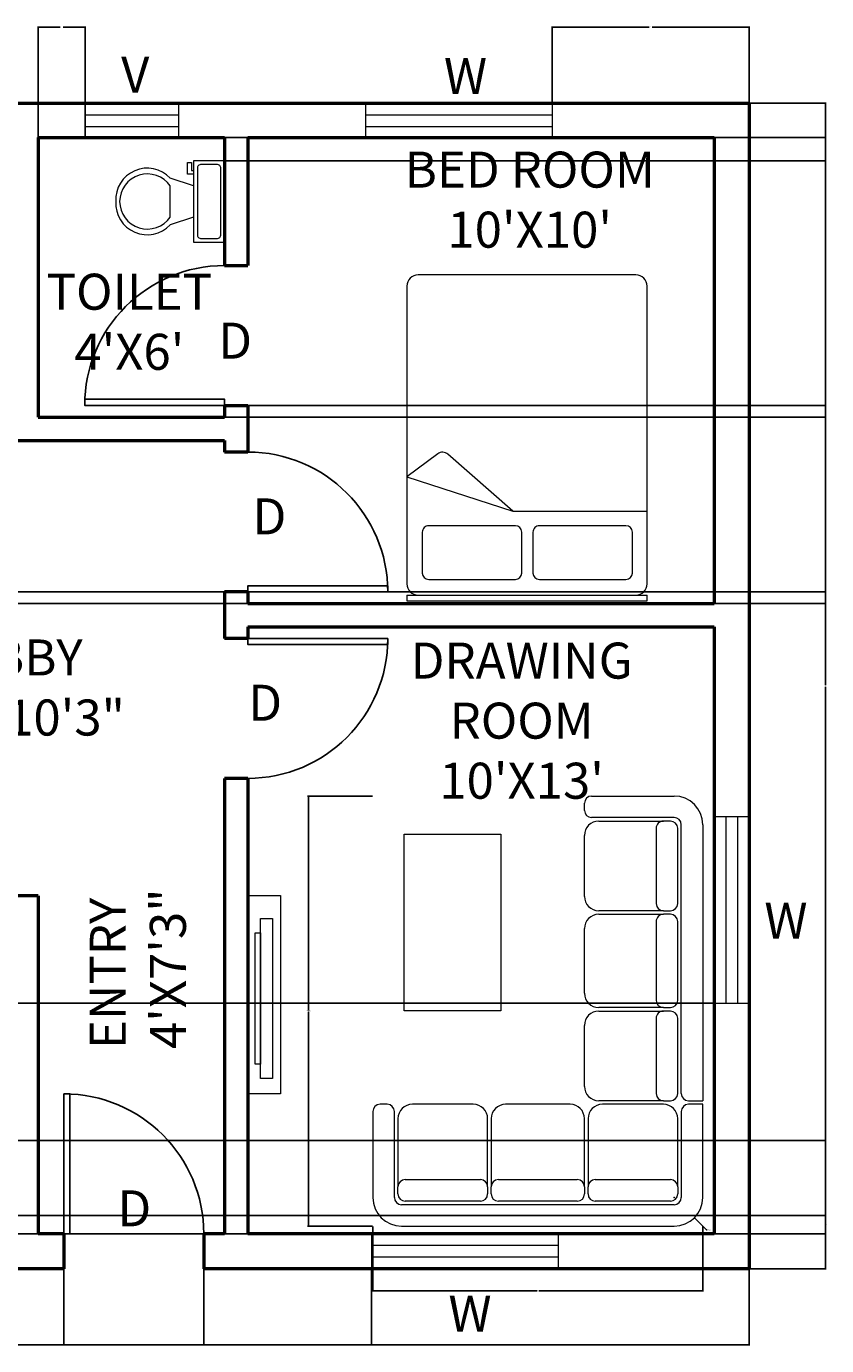
# Model space of a CAD drawing. Units: inches. Extents: x 1916 to 2328, y 785 to 1125.
# Tile 3 of 3: x 2122 to 2328, y 785 to 1125. Entities that reach past the tile are written whole.
import ezdxf

# ---------------------------------------------------------------- set-up
doc = ezdxf.new("R2010")
doc.units = ezdxf.units.IN
for name, color, linetype, lineweight in [('A-ANNO-DIMS', 2, 'Continuous', 18), ('A-ANNO-TEXT', 7, 'Continuous', 18), ('A-AREA-IDEN', 7, 'Continuous', 25), ('A-DOOR', 3, 'Continuous', 25), ('A-FLOR-FIXT', 9, 'Continuous', 18), ('A-FURN', 8, 'Continuous', 18), ('A-GLAZ', 4, 'Continuous', 18), ('A-WALL', 7, 'Continuous', 50)]:
    doc.layers.add(name, color=color, linetype=linetype, lineweight=lineweight)
doc.styles.get("Standard").update_dxf_attribs({"font": 'arial.ttf'})
doc.dimstyles.get("Standard").update_dxf_attribs({"dimtxt": 0.18, "dimasz": 0.18, "dimexe": 0.18, "dimexo": 0.0625, "dimgap": 0.09, "dimtad": 0, "dimtih": 1, "dimtoh": 1, "dimdec": 4, "dimzin": 0, "dimdsep": 46, "dimtxsty": 'Standard', "dimcen": 0.09, "dimadec": 0, "dimazin": 0, "dimtfac": 1, "dimtdec": 4, "dimtofl": 0, "dimtmove": 0, "dimatfit": 3, "dimfxl": 1, "dimtolj": 1, "dimtzin": 0, "dimarcsym": 0})

# ---------------------------------------------------------------- blocks, each defined once
blk = doc.blocks.new('*U2')
for p, q in [((0, 0), (0, -6)), ((40, 0), (40, -6))]:
    blk.add_line(p, q)
blk.add_lwpolyline([(0, 0), (0, 40), (1.75, 40), (1.75, 0)], close=True)
blk.add_arc((0, 0), 40, 0, 90)
blk = doc.blocks.new('*U3')
for p, q in [((0, 0), (0, 6)), ((40, 0), (40, 6))]:
    blk.add_line(p, q)
blk.add_lwpolyline([(0, 0), (0, -40), (1.75, -40), (1.75, 0)], close=True)
blk.add_arc((0, 0), 40, 270, 0)
blk = doc.blocks.new('A$C2AFA021D')
for p, q in [((0.8, 2.3), (0.2, 2.3)), ((0.85, 2.2), (0.85, 2.25)), ((0.2, 2.15), (0.8, 2.15)), ((0.225, 2.125), (0.275, 2.125)), ((0.75, 2.125), (0.275, 2.125)), ((0, 2.1), (0, 0.2)), ((0.15, 0.2), (0.15, 2.1)), ((0.175, 1.55), (0.175, 2.075)), ((0.325, 2.075), (0.325, 1.55)), ((0.85, 1.6), (0.85, 2.025)), ((0.275, 1.5), (0.225, 1.5)), ((0.225, 1.475), (0.275, 1.475)), ((0.275, 1.5), (0.75, 1.5)), ((0.75, 1.475), (0.275, 1.475)), ((0.175, 0.875), (0.175, 1.425)), ((0.325, 1.425), (0.325, 0.875)), ((0.85, 0.925), (0.85, 1.375)), ((0.175, 0.225), (0.175, 0.75)), ((0.275, 0.825), (0.225, 0.825)), ((0.225, 0.8), (0.275, 0.8)), ((0.275, 0.825), (0.75, 0.825)), ((0.75, 0.8), (0.275, 0.8)), ((0.325, 0.75), (0.325, 0.225)), ((0.975, 0.825), (1.4, 0.825)), ((1.625, 0.825), (2.075, 0.825)), ((2.3, 0.825), (2.725, 0.825)), ((2.85, 0.2), (2.85, 0.775)), ((2.9, 0.825), (2.95, 0.825)), ((3, 0.775), (3, 0.2)), ((0.85, 0.275), (0.85, 0.7)), ((0.875, 0.275), (0.875, 0.725)), ((1.5, 0.725), (1.5, 0.275)), ((1.525, 0.275), (1.525, 0.725)), ((2.175, 0.725), (2.175, 0.275)), ((2.2, 0.275), (2.2, 0.725)), ((2.825, 0.725), (2.825, 0.275)), ((1.45, 0.325), (0.925, 0.325)), ((2.125, 0.325), (1.575, 0.325)), ((2.775, 0.325), (2.25, 0.325)), ((0.875, 0.275), (0.875, 0.225)), ((1.5, 0.225), (1.5, 0.275)), ((1.525, 0.275), (1.525, 0.225)), ((2.175, 0.225), (2.175, 0.275)), ((2.2, 0.275), (2.2, 0.225)), ((2.825, 0.225), (2.825, 0.275)), ((0.8, 0.15), (0.2, 0.15)), ((0.275, 0.175), (0.225, 0.175)), ((0.275, 0.175), (0.75, 0.175)), ((0.85, 0), (0.85, 0.1)), ((0.875, 0.1), (0.875, 0)), ((0.925, 0.175), (1.45, 0.175)), ((0.925, 0.15), (2.8, 0.15)), ((1.575, 0.175), (2.125, 0.175)), ((2.25, 0.175), (2.775, 0.175)), ((0.2, 0), (0.85, 0)), ((2.8, 0), (0.875, 0))]:
    blk.add_line(p, q)
for centre, radius, start, end in [((0.2, 2.1), 0.2, 90, 180), ((0.8, 2.25), 0.05, 0, 90), ((0.2, 2.1), 0.05, 90, 180), ((0.225, 2.075), 0.05, 90, 180), ((0.275, 2.075), 0.05, 0, 90), ((0.75, 2.025), 0.1, 0, 90), ((0.8, 2.2), 0.05, 270, 0), ((0.75, 1.6), 0.1, 270, 0), ((0.225, 1.55), 0.05, 180, 270), ((0.225, 1.425), 0.05, 90, 180), ((0.275, 1.55), 0.05, 270, 0), ((0.275, 1.425), 0.05, 0, 90), ((0.75, 1.375), 0.1, 360, 90), ((0.75, 0.925), 0.1, 270, 0), ((0.225, 0.875), 0.05, 180, 270), ((0.275, 0.875), 0.05, 270, 0), ((0.225, 0.75), 0.05, 90, 180), ((0.275, 0.75), 0.05, 0, 90), ((0.75, 0.7), 0.1, 0, 90), ((0.975, 0.725), 0.1, 90, 180), ((1.4, 0.725), 0.1, 0, 90), ((1.625, 0.725), 0.1, 90, 180), ((2.075, 0.725), 0.1, 0, 90), ((2.3, 0.725), 0.1, 90, 180), ((2.725, 0.725), 0.1, 0, 90), ((2.9, 0.775), 0.05, 90, 180), ((2.95, 0.775), 0.05, 0, 90), ((0.925, 0.275), 0.05, 90, 180), ((1.45, 0.275), 0.05, 360, 90), ((1.575, 0.275), 0.05, 90, 180), ((2.125, 0.275), 0.05, 360, 90), ((2.25, 0.275), 0.05, 90, 180), ((2.775, 0.275), 0.05, 360, 90), ((0.2, 0.2), 0.2, 180, 270), ((0.2, 0.2), 0.05, 180, 270), ((0.225, 0.225), 0.05, 180, 270), ((0.275, 0.225), 0.05, 270, 0), ((0.75, 0.275), 0.1, 270, 0), ((0.925, 0.225), 0.05, 180, 270), ((1.45, 0.225), 0.05, 270, 0), ((1.575, 0.225), 0.05, 180, 270), ((2.125, 0.225), 0.05, 270, 0), ((2.25, 0.225), 0.05, 180, 270), ((2.775, 0.225), 0.05, 270, 0), ((2.8, 0.2), 0.2, 270, 0), ((2.8, 0.2), 0.05, 270, 0), ((0.8, 0.1), 0.05, 0, 90), ((0.925, 0.1), 0.05, 90, 180)]:
    blk.add_arc(centre, radius, start, end)
blk = doc.blocks.new('A$C164346CA')
for p, q in [((0, 2.035), (0, 2)), ((1.5, 2.035), (0, 2.035)), ((1.5, 2), (0, 2)), ((1.5, 2), (1.5, 2.035)), ((0, 1.93), (0, 0.07)), ((0.6731, 1.9024), (0.1319, 1.9024)), ((1.364, 1.9024), (0.8228, 1.9024)), ((1.5, 0.07), (1.5, 1.93)), ((0.0919, 1.8624), (0.0919, 1.6069)), ((0.7131, 1.6069), (0.7131, 1.8624)), ((0.7828, 1.8624), (0.7828, 1.6069)), ((1.404, 1.6069), (1.404, 1.8624)), ((0.1319, 1.5669), (0.6731, 1.5669)), ((0.8228, 1.5669), (1.364, 1.5669)), ((0.8395, 1.4761), (0, 1.4761)), ((0.8395, 1.4761), (1.2448, 1.12)), ((1.5, 1.2611), (0.8395, 1.4761)), ((1.3077, 1.1175), (1.5, 1.2611)), ((0.07, 0), (1.43, 0))]:
    blk.add_line(p, q)
for centre, radius, start, end in [((0.07, 1.93), 0.07, 90, 180), ((1.43, 1.93), 0.07, 0, 90), ((0.1319, 1.8624), 0.04, 90, 180), ((0.6731, 1.8624), 0.04, 0, 90), ((0.8228, 1.8624), 0.04, 90, 180), ((1.364, 1.8624), 0.04, 0, 90), ((0.1319, 1.6069), 0.04, 180, 270), ((0.6731, 1.6069), 0.04, 270, 0), ((0.8228, 1.6069), 0.04, 180, 270), ((1.364, 1.6069), 0.04, 270, 0), ((1.2778, 1.1575), 0.05, 228.69584, 306.75789), ((0.07, 0.07), 0.07, 180, 270), ((1.43, 0.07), 0.07, 270, 0)]:
    blk.add_arc(centre, radius, start, end)
blk = doc.blocks.new('*U10')
for p, q in [((9.5, -6), (9.5, -2)), ((-10, -8.5), (-8, -8.5)), ((-10, -9.5), (-10, -8.5)), ((-7, -9.5), (-10, -9.5)), ((-8, -8.5), (-8, -8)), ((-7, -8), (-7, -9.5)), ((-4, -8), (-6, -14)), ((4, -8), (6, -14)), ((4, -14), (-4, -14))]:
    blk.add_line(p, q)
blk.add_lwpolyline([(10.5, -8), (10.5, 0), (-10.5, 0), (-10.5, -8)], close=True)
for points in [[(-9.5, -2), (-9.5, -6)], [(8.5, -1), (-8.5, -1)], [(-8.5, -7), (8.5, -7)]]:
    blk.add_lwpolyline(points)
for centre, radius, start, end in [((-8.625, -1.875), 0.8839, 81.8699, 188.1301), ((8.625, -1.875), 0.8839, 351.8699, 98.1301), ((-8.625, -6.125), 0.8839, 171.869898, 278.1301), ((8.625, -6.125), 0.8839, 261.8699, 8.1301), ((-0.4772, -19.9188), 8.0953, 133.01722, 273.38), ((0.0374, -19.8731), 7.127, 124.50543, 269.7), ((-0.0373, -19.8731), 7.127, 270.3, 55.4946), ((0.4773, -19.9188), 8.0953, 266.62, 46.9828)]:
    blk.add_arc(centre, radius, start, end)
blk = doc.blocks.new('WIN-48-JAMB-9')
for p, q in [((0, 9), (0, 0)), ((48, 9), (48, 0)), ((48, 6), (0, 6)), ((48, 3), (0, 3))]:
    blk.add_line(p, q)
blk = doc.blocks.new('WIN-48-JAMB-8_78')
for p, q in [((0, 8.78), (0, 0)), ((48, 8.78), (48, 0)), ((0, 5.78), (48, 5.78)), ((0, 2.78), (48, 2.78))]:
    blk.add_line(p, q)
blk = doc.blocks.new('VENT-24')
for p, q in [((0, 8.78), (0, 0)), ((24, 8.78), (24, 0)), ((0, 5.78), (24, 5.78)), ((0, 2.78), (24, 2.78))]:
    blk.add_line(p, q)
blk = doc.blocks.new('*D29')
at = {"layer": 'A-ANNO-DIMS', "color": 0, "lineweight": -2, "transparency": 16777216}
for p, q in [((2211.34, 926.56), (2194.61, 926.56)), ((2194.79, 926.38), (2194.79, 871.37)), ((2194.79, 816), (2194.79, 871.01)), ((2211.34, 815.82), (2194.61, 815.82))]:
    blk.add_line(p, q, dxfattribs=at)
at = {"layer": 'A-ANNO-DIMS', "color": 0, "transparency": 16777216}
for points in [[(2194.76, 926.38), (2194.82, 926.38), (2194.79, 926.56)], [(2194.76, 816), (2194.82, 816), (2194.79, 815.82)]]:
    blk.add_solid(points, dxfattribs=at)
at = {"layer": 'Defpoints', "color": 0, "transparency": 16777216}
for p in [(2194.79, 926.56), (2211.4, 926.56), (2211.4, 815.82)]:
    blk.add_point(p, dxfattribs=at)
at = {"layer": 'A-ANNO-DIMS', "color": 0, "transparency": 16777216, "insert": (2194.79, 871.19), "char_height": 0.18, "attachment_point": 5}
blk.add_mtext('\\A1;SOFA 111', dxfattribs=at)
blk = doc.blocks.new('*D30')
at = {"layer": 'A-ANNO-DIMS', "color": 0, "lineweight": -2, "transparency": 16777216}
for p, q in [((2211.4, 815.76), (2211.4, 799.03)), ((2296.29, 815.76), (2296.29, 799.03)), ((2211.58, 799.21), (2253.63, 799.21)), ((2296.11, 799.21), (2254.07, 799.21))]:
    blk.add_line(p, q, dxfattribs=at)
at = {"layer": 'A-ANNO-DIMS', "color": 0, "transparency": 16777216}
for points in [[(2211.58, 799.24), (2211.58, 799.18), (2211.4, 799.21)], [(2296.11, 799.24), (2296.11, 799.18), (2296.29, 799.21)]]:
    blk.add_solid(points, dxfattribs=at)
at = {"layer": 'Defpoints', "color": 0, "transparency": 16777216}
for p in [(2211.4, 815.82), (2296.29, 815.82), (2211.4, 799.21)]:
    blk.add_point(p, dxfattribs=at)
at = {"layer": 'A-ANNO-DIMS', "color": 0, "transparency": 16777216, "insert": (2253.85, 799.21), "char_height": 0.18, "attachment_point": 5}
blk.add_mtext('\\A1;85', dxfattribs=at)
blk = doc.blocks.new('*D33')
at = {"layer": 'A-ANNO-DIMS', "color": 0, "lineweight": -2, "transparency": 16777216}
for p, q in [((2125.23, 1096.16), (2125.23, 1124.67)), ((2125.41, 1124.49), (2130.91, 1124.49)), ((2137.17, 1124.49), (2131.68, 1124.49)), ((2137.35, 1096.16), (2137.35, 1124.67))]:
    blk.add_line(p, q, dxfattribs=at)
at = {"layer": 'A-ANNO-DIMS', "color": 0, "transparency": 16777216}
for points in [[(2125.41, 1124.52), (2125.41, 1124.46), (2125.23, 1124.49)], [(2137.17, 1124.52), (2137.17, 1124.46), (2137.35, 1124.49)]]:
    blk.add_solid(points, dxfattribs=at)
at = {"layer": 'Defpoints', "color": 0, "transparency": 16777216}
for p in [(2137.35, 1124.49), (2125.23, 1096.1), (2137.35, 1096.1)]:
    blk.add_point(p, dxfattribs=at)
at = {"layer": 'A-ANNO-DIMS', "color": 0, "transparency": 16777216, "insert": (2131.29, 1124.49), "char_height": 0.18, "attachment_point": 5}
blk.add_mtext('\\A1;12.12', dxfattribs=at)
blk = doc.blocks.new('*D34')
at = {"layer": 'A-ANNO-DIMS', "color": 0, "lineweight": -2, "transparency": 16777216}
for p, q in [((2257.52, 1104.94), (2257.52, 1124.67)), ((2257.7, 1124.49), (2282.48, 1124.49)), ((2308.05, 1124.49), (2283.27, 1124.49)), ((2308.23, 1104.94), (2308.23, 1124.67))]:
    blk.add_line(p, q, dxfattribs=at)
at = {"layer": 'A-ANNO-DIMS', "color": 0, "transparency": 16777216}
for points in [[(2257.7, 1124.52), (2257.7, 1124.46), (2257.52, 1124.49)], [(2308.05, 1124.52), (2308.05, 1124.46), (2308.23, 1124.49)]]:
    blk.add_solid(points, dxfattribs=at)
at = {"layer": 'Defpoints', "color": 0, "transparency": 16777216}
for p in [(2308.23, 1124.49), (2257.52, 1104.88), (2308.23, 1104.88)]:
    blk.add_point(p, dxfattribs=at)
at = {"layer": 'A-ANNO-DIMS', "color": 0, "transparency": 16777216, "insert": (2282.88, 1124.49), "char_height": 0.18, "attachment_point": 5}
blk.add_mtext('\\A1;50.72', dxfattribs=at)
blk = doc.blocks.new('*D36')
at = {"layer": 'A-ANNO-DIMS', "color": 0, "lineweight": -2, "transparency": 16777216}
for p, q in [((2299.17, 873.26), (1916.44, 873.26)), ((1916.62, 873.08), (1916.62, 843.75)), ((1916.62, 814.06), (1916.62, 843.39)), ((2299.17, 813.88), (1916.44, 813.88))]:
    blk.add_line(p, q, dxfattribs=at)
at = {"layer": 'A-ANNO-DIMS', "color": 0, "transparency": 16777216}
for points in [[(1916.59, 873.08), (1916.65, 873.08), (1916.62, 873.26)], [(1916.59, 814.06), (1916.65, 814.06), (1916.62, 813.88)]]:
    blk.add_solid(points, dxfattribs=at)
at = {"layer": 'Defpoints', "color": 0, "transparency": 16777216}
for p in [(1916.62, 873.26), (2299.23, 873.26), (2299.23, 813.88)]:
    blk.add_point(p, dxfattribs=at)
at = {"layer": 'A-ANNO-DIMS', "color": 0, "transparency": 16777216, "insert": (1916.62, 843.57), "char_height": 0.18, "attachment_point": 5}
blk.add_mtext('\\A1;59.38', dxfattribs=at)
blk = doc.blocks.new('*D37')
at = {"layer": 'A-ANNO-DIMS', "color": 0, "lineweight": -2, "transparency": 16777216}
for p, q in [((2119.23, 804.82), (2119.23, 785.08)), ((2131.87, 804.82), (2131.87, 785.08)), ((2119.41, 785.26), (2125.1, 785.26)), ((2131.69, 785.26), (2126.01, 785.26))]:
    blk.add_line(p, q, dxfattribs=at)
at = {"layer": 'A-ANNO-DIMS', "color": 0, "transparency": 16777216}
for points in [[(2119.41, 785.29), (2119.41, 785.23), (2119.23, 785.26)], [(2131.69, 785.29), (2131.69, 785.23), (2131.87, 785.26)]]:
    blk.add_solid(points, dxfattribs=at)
at = {"layer": 'Defpoints', "color": 0, "transparency": 16777216}
for p in [(2119.23, 804.88), (2131.87, 804.88), (2131.87, 785.26)]:
    blk.add_point(p, dxfattribs=at)
at = {"layer": 'A-ANNO-DIMS', "color": 0, "transparency": 16777216, "insert": (2125.55, 785.26), "char_height": 0.18, "attachment_point": 5}
blk.add_mtext('\\A1;12.642', dxfattribs=at)
blk = doc.blocks.new('*D38')
at = {"layer": 'A-ANNO-DIMS', "color": 0, "lineweight": -2, "transparency": 16777216}
for p, q in [((2131.87, 804.82), (2131.87, 785.08)), ((2167.87, 804.82), (2167.87, 785.08)), ((2132.05, 785.26), (2149.66, 785.26)), ((2167.69, 785.26), (2150.09, 785.26))]:
    blk.add_line(p, q, dxfattribs=at)
at = {"layer": 'A-ANNO-DIMS', "color": 0, "transparency": 16777216}
for points in [[(2132.05, 785.29), (2132.05, 785.23), (2131.87, 785.26)], [(2167.69, 785.29), (2167.69, 785.23), (2167.87, 785.26)]]:
    blk.add_solid(points, dxfattribs=at)
at = {"layer": 'Defpoints', "color": 0, "transparency": 16777216}
for p in [(2131.87, 804.88), (2167.87, 804.88), (2167.87, 785.26)]:
    blk.add_point(p, dxfattribs=at)
at = {"layer": 'A-ANNO-DIMS', "color": 0, "transparency": 16777216, "insert": (2149.87, 785.26), "char_height": 0.18, "attachment_point": 5}
blk.add_mtext('\\A1;36', dxfattribs=at)
blk = doc.blocks.new('*D39')
at = {"layer": 'A-ANNO-DIMS', "color": 0, "lineweight": -2, "transparency": 16777216}
for p, q in [((2167.87, 804.82), (2167.87, 785.08)), ((2211.05, 804.82), (2211.05, 785.08)), ((2168.05, 785.26), (2189.06, 785.26)), ((2210.87, 785.26), (2189.86, 785.26))]:
    blk.add_line(p, q, dxfattribs=at)
at = {"layer": 'A-ANNO-DIMS', "color": 0, "transparency": 16777216}
for points in [[(2168.05, 785.29), (2168.05, 785.23), (2167.87, 785.26)], [(2210.87, 785.29), (2210.87, 785.23), (2211.05, 785.26)]]:
    blk.add_solid(points, dxfattribs=at)
at = {"layer": 'Defpoints', "color": 0, "transparency": 16777216}
for p in [(2167.87, 804.88), (2211.05, 804.88), (2211.05, 785.26)]:
    blk.add_point(p, dxfattribs=at)
at = {"layer": 'A-ANNO-DIMS', "color": 0, "transparency": 16777216, "insert": (2189.46, 785.26), "char_height": 0.18, "attachment_point": 5}
blk.add_mtext('\\A1;43.17', dxfattribs=at)
blk = doc.blocks.new('*D41')
at = {"layer": 'A-ANNO-DIMS', "color": 0, "lineweight": -2, "transparency": 16777216}
for p, q in [((2065.3, 837.88), (2328.03, 837.88)), ((2327.85, 837.7), (2327.85, 826.06)), ((2327.85, 814.06), (2327.85, 825.7)), ((2065.3, 813.88), (2328.03, 813.88))]:
    blk.add_line(p, q, dxfattribs=at)
at = {"layer": 'A-ANNO-DIMS', "color": 0, "transparency": 16777216}
for points in [[(2327.82, 837.7), (2327.88, 837.7), (2327.85, 837.88)], [(2327.82, 814.06), (2327.88, 814.06), (2327.85, 813.88)]]:
    blk.add_solid(points, dxfattribs=at)
at = {"layer": 'Defpoints', "color": 0, "transparency": 16777216}
for p in [(2065.23, 837.88), (2327.85, 837.88), (2065.23, 813.88)]:
    blk.add_point(p, dxfattribs=at)
at = {"layer": 'A-ANNO-DIMS', "color": 0, "transparency": 16777216, "insert": (2327.85, 825.88), "char_height": 0.18, "attachment_point": 5}
blk.add_mtext('\\A1;24', dxfattribs=at)
blk = doc.blocks.new('*D45')
at = {"layer": 'A-ANNO-DIMS', "color": 0, "lineweight": -2, "transparency": 16777216}
for p, q in [((2044.13, 818.58), (2328.03, 818.58)), ((2327.85, 818.4), (2327.85, 816.41)), ((2327.85, 814.06), (2327.85, 816.05)), ((2065.3, 813.88), (2328.03, 813.88))]:
    blk.add_line(p, q, dxfattribs=at)
at = {"layer": 'A-ANNO-DIMS', "color": 0, "transparency": 16777216}
for points in [[(2327.82, 818.4), (2327.88, 818.4), (2327.85, 818.58)], [(2327.82, 814.06), (2327.88, 814.06), (2327.85, 813.88)]]:
    blk.add_solid(points, dxfattribs=at)
at = {"layer": 'Defpoints', "color": 0, "transparency": 16777216}
for p in [(2044.07, 818.58), (2065.23, 813.88), (2327.85, 813.88)]:
    blk.add_point(p, dxfattribs=at)
at = {"layer": 'A-ANNO-DIMS', "color": 0, "transparency": 16777216, "insert": (2327.85, 816.23), "char_height": 0.18, "attachment_point": 5}
blk.add_mtext('\\A1;4.702', dxfattribs=at)
blk = doc.blocks.new('*D49')
at = {"layer": 'A-ANNO-DIMS', "color": 0, "lineweight": -2, "transparency": 16777216}
for p, q in [((2173.3, 1096.1), (2328.03, 1096.1)), ((2327.85, 1095.92), (2327.85, 1093.28)), ((2173.3, 1090.1), (2328.03, 1090.1)), ((2327.85, 1090.28), (2327.85, 1092.92))]:
    blk.add_line(p, q, dxfattribs=at)
at = {"layer": 'A-ANNO-DIMS', "color": 0, "transparency": 16777216}
for points in [[(2327.82, 1095.92), (2327.88, 1095.92), (2327.85, 1096.1)], [(2327.82, 1090.28), (2327.88, 1090.28), (2327.85, 1090.1)]]:
    blk.add_solid(points, dxfattribs=at)
at = {"layer": 'Defpoints', "color": 0, "transparency": 16777216}
for p in [(2173.23, 1096.1), (2327.85, 1096.1), (2173.23, 1090.1)]:
    blk.add_point(p, dxfattribs=at)
at = {"layer": 'A-ANNO-DIMS', "color": 0, "transparency": 16777216, "insert": (2327.85, 1093.1), "char_height": 0.18, "attachment_point": 5}
blk.add_mtext('\\A1;6', dxfattribs=at)
blk = doc.blocks.new('*D52')
at = {"layer": 'A-ANNO-DIMS', "color": 0, "lineweight": -2, "transparency": 16777216}
for p, q in [((2173.3, 1027.1), (2328.03, 1027.1)), ((2327.85, 1026.92), (2327.85, 1025.78)), ((2173.3, 1024.1), (2328.03, 1024.1)), ((2327.85, 1024.28), (2327.85, 1025.42))]:
    blk.add_line(p, q, dxfattribs=at)
at = {"layer": 'A-ANNO-DIMS', "color": 0, "transparency": 16777216}
for points in [[(2327.82, 1026.92), (2327.88, 1026.92), (2327.85, 1027.1)], [(2327.82, 1024.28), (2327.88, 1024.28), (2327.85, 1024.1)]]:
    blk.add_solid(points, dxfattribs=at)
at = {"layer": 'Defpoints', "color": 0, "transparency": 16777216}
for p in [(2173.23, 1027.1), (2327.85, 1027.1), (2173.23, 1024.1)]:
    blk.add_point(p, dxfattribs=at)
at = {"layer": 'A-ANNO-DIMS', "color": 0, "transparency": 16777216, "insert": (2327.85, 1025.6), "char_height": 0.18, "attachment_point": 5}
blk.add_mtext('\\A1;3', dxfattribs=at)
blk = doc.blocks.new('*D54')
at = {"layer": 'A-ANNO-DIMS', "color": 0, "lineweight": -2, "transparency": 16777216}
for p, q in [((2065.3, 979.1), (2328.03, 979.1)), ((2327.85, 978.92), (2327.85, 977.78)), ((2065.3, 976.1), (2328.03, 976.1)), ((2327.85, 976.28), (2327.85, 977.42))]:
    blk.add_line(p, q, dxfattribs=at)
at = {"layer": 'A-ANNO-DIMS', "color": 0, "transparency": 16777216}
for points in [[(2327.82, 978.92), (2327.88, 978.92), (2327.85, 979.1)], [(2327.82, 976.28), (2327.88, 976.28), (2327.85, 976.1)]]:
    blk.add_solid(points, dxfattribs=at)
at = {"layer": 'Defpoints', "color": 0, "transparency": 16777216}
for p in [(2065.23, 979.1), (2327.85, 979.1), (2065.23, 976.1)]:
    blk.add_point(p, dxfattribs=at)
at = {"layer": 'A-ANNO-DIMS', "color": 0, "transparency": 16777216, "insert": (2327.85, 977.6), "char_height": 0.18, "attachment_point": 5}
blk.add_mtext('\\A1;3', dxfattribs=at)
blk = doc.blocks.new('*D57')
at = {"layer": 'A-ANNO-DIMS', "color": 0, "lineweight": -2, "transparency": 16777216}
for p, q in [((1936.23, 804.82), (1936.23, 785.08)), ((2308.23, 804.82), (2308.23, 785.08)), ((1936.41, 785.26), (2121.95, 785.26)), ((2308.05, 785.26), (2122.52, 785.26))]:
    blk.add_line(p, q, dxfattribs=at)
at = {"layer": 'A-ANNO-DIMS', "color": 0, "transparency": 16777216}
for points in [[(1936.41, 785.29), (1936.41, 785.23), (1936.23, 785.26)], [(2308.05, 785.29), (2308.05, 785.23), (2308.23, 785.26)]]:
    blk.add_solid(points, dxfattribs=at)
at = {"layer": 'Defpoints', "color": 0, "transparency": 16777216}
for p in [(1936.23, 804.88), (2308.23, 804.88), (2308.23, 785.26)]:
    blk.add_point(p, dxfattribs=at)
at = {"layer": 'A-ANNO-DIMS', "color": 0, "transparency": 16777216, "insert": (2122.23, 785.26), "char_height": 0.18, "attachment_point": 5}
blk.add_mtext('\\A1;372', dxfattribs=at)
blk = doc.blocks.new('*D58')
at = {"layer": 'A-ANNO-DIMS', "color": 0, "lineweight": -2, "transparency": 16777216}
for p, q in [((2308.3, 1104.88), (2328.03, 1104.88)), ((2327.85, 1104.7), (2327.85, 955.06)), ((2327.85, 805.06), (2327.85, 954.7)), ((2308.3, 804.88), (2328.03, 804.88))]:
    blk.add_line(p, q, dxfattribs=at)
at = {"layer": 'A-ANNO-DIMS', "color": 0, "transparency": 16777216}
for points in [[(2327.82, 1104.7), (2327.88, 1104.7), (2327.85, 1104.88)], [(2327.82, 805.06), (2327.88, 805.06), (2327.85, 804.88)]]:
    blk.add_solid(points, dxfattribs=at)
at = {"layer": 'Defpoints', "color": 0, "transparency": 16777216}
for p in [(2308.23, 1104.88), (2327.85, 1104.88), (2308.23, 804.88)]:
    blk.add_point(p, dxfattribs=at)
at = {"layer": 'A-ANNO-DIMS', "color": 0, "transparency": 16777216, "insert": (2327.85, 954.88), "char_height": 0.18, "attachment_point": 5}
blk.add_mtext('\\A1;300', dxfattribs=at)
blk = doc.blocks.new('*D59')
at = {"layer": 'A-ANNO-DIMS', "color": 0, "lineweight": -2, "transparency": 16777216}
for p, q in [((2288.82, 823.21), (2289, 823.21)), ((2288.91, 823.12), (2288.91, 823.3)), ((2297.26, 814.85), (2294.26, 817.86)), ((2297.44, 814.85), (2297.26, 814.85))]:
    blk.add_line(p, q, dxfattribs=at)
at = {"layer": 'A-ANNO-DIMS', "color": 0, "transparency": 16777216}
blk.add_solid([(2294.28, 817.88), (2294.24, 817.84), (2294.13, 817.99)], dxfattribs=at)
at = {"layer": 'Defpoints', "color": 0, "transparency": 16777216}
for p in [(2288.91, 823.21), (2294.13, 817.99)]:
    blk.add_point(p, dxfattribs=at)
at = {"layer": 'A-ANNO-DIMS', "color": 0, "transparency": 16777216, "insert": (2298.12, 814.85), "char_height": 0.18, "attachment_point": 5}
blk.add_mtext('\\A1;3X R7.382', dxfattribs=at)

msp = doc.modelspace()

# ---------------------------------------------------------------- linework, layer by layer
at = {"layer": 'A-FURN'}
for p, q in [((2219.4173, 916.6997), (2244.365, 916.6997)), ((2219.4173, 871.2769), (2219.4173, 916.6997)), ((2244.365, 916.6997), (2244.365, 871.2769)), ((2179.2334, 900.9304), (2187.6578, 900.9304)), ((2187.6578, 900.9304), (2187.6578, 849.8636)), ((2244.365, 871.2769), (2219.4173, 871.2769)), ((2187.6578, 849.8636), (2179.2334, 849.8636))]:
    msp.add_line(p, q, dxfattribs=at)
for points in [[(2182.4578, 895.0669), (2185.56, 895.0669), (2185.56, 853.8864), (2182.4578, 853.8864)], [(2181.1283, 891.3031), (2182.4578, 891.3031), (2182.4578, 857.5395), (2181.1283, 857.5395)]]:
    msp.add_lwpolyline(points, close=True, dxfattribs=at)
at = {"layer": 'A-WALL'}
for p, q in [((1936.2334, 1104.8797), (2308.2334, 1104.8797)), ((2308.2334, 1104.8797), (2308.2334, 804.8797)), ((2125.2334, 1096.1011), (2125.2334, 1024.1011)), ((2125.2334, 1096.1011), (2173.2334, 1096.1011)), ((2173.2334, 1096.1011), (2173.2334, 1063.1011)), ((2179.2334, 1096.1011), (2179.2334, 1063.1011)), ((2179.2334, 1096.1011), (2299.2334, 1096.1011)), ((2299.2334, 1096.1011), (2299.2334, 976.1011)), ((2173.2334, 1063.1011), (2179.2334, 1063.1011)), ((2173.2334, 1027.1011), (2179.2334, 1027.1011)), ((2173.2334, 1027.1011), (2173.2334, 1024.1011)), ((2179.2334, 1027.1011), (2179.2334, 1015.1011)), ((2125.2334, 1024.1011), (2173.2334, 1024.1011)), ((2116.2334, 1018.1011), (2173.2334, 1018.1011)), ((2173.2334, 1018.1011), (2173.2334, 1015.1011)), ((2179.2334, 1015.1011), (2173.2334, 1015.1011)), ((2179.2334, 979.1011), (2173.2334, 979.1011)), ((2173.2334, 979.1011), (2173.2334, 967.1011)), ((2179.2334, 979.1011), (2179.2334, 976.1011)), ((2179.2334, 976.1011), (2299.2334, 976.1011)), ((2179.2334, 970.1011), (2299.2334, 970.1011)), ((2179.2334, 970.1011), (2179.2334, 967.1011)), ((2299.2334, 970.1011), (2299.2334, 813.8797)), ((2179.2334, 967.1011), (2173.2334, 967.1011)), ((2179.2334, 931.1011), (2173.2334, 931.1011)), ((2173.2334, 931.1011), (2173.2334, 813.8797)), ((2179.2334, 931.1011), (2179.2334, 813.8797)), ((2125.2334, 900.8797), (2065.2334, 900.8797)), ((2125.2334, 900.8797), (2125.2334, 813.8797)), ((2131.8749, 813.8797), (2125.2334, 813.8797)), ((2131.8749, 813.8797), (2131.8749, 804.8797)), ((2173.2334, 813.8797), (2167.8749, 813.8797)), ((2167.8749, 813.8797), (2167.8749, 804.8797)), ((2299.2334, 813.8797), (2179.2334, 813.8797)), ((2131.8749, 804.8797), (1936.2334, 804.8797)), ((2308.2334, 804.8797), (2167.8749, 804.8797))]:
    msp.add_line(p, q, dxfattribs=at)

# ---------------------------------------------------------------- block references
at = {"layer": 'A-DOOR'}
for name, p, xscale, yscale, zscale, rotation in [('*U2', (2173.2334, 1027.1011), 0.9, 0.9, 0.9, 90), ('*U3', (2179.2334, 979.1011), 0.9, 0.9, 0.9, 90), ('*U2', (2179.2334, 967.1011), 0.900000000000003, 0.900000000000003, 0.900000000000003, 270)]:
    msp.add_blockref(name, p, dxfattribs=dict(at, xscale=xscale, yscale=yscale, zscale=zscale, rotation=rotation))
at = {"layer": 'A-DOOR', "xscale": 0.8999999999999889, "yscale": 0.8999999999999889, "zscale": 0.8999999999999889}
msp.add_blockref('*U2', (2131.8749, 813.8797), dxfattribs=at)
at = {"layer": 'A-FLOR-FIXT', "rotation": 270}
msp.add_blockref('*U10', (2173.2334, 1079.6011), dxfattribs=at)
at = {"layer": 'A-FURN'}
for name, p, xscale, yscale, zscale, rotation in [('A$C164346CA', (2281.9663, 1060.6864), 41.2001878286395, 41.2001878286395, 41.2001878286395, 180), ('A$C2AFA021D', (2296.2937, 815.8242), 36.91064245516507, 36.91064245516507, 36.91064245516507, 90)]:
    msp.add_blockref(name, p, dxfattribs=dict(at, xscale=xscale, yscale=yscale, zscale=zscale, rotation=rotation))
at = {"layer": 'A-GLAZ'}
for name, p in [('VENT-24', (2137.3543, 1096.1011)), ('WIN-48-JAMB-8_78', (2209.5169, 1096.1011)), ('WIN-48-JAMB-9', (2211.047, 804.8797))]:
    msp.add_blockref(name, p, dxfattribs=at)
at = {"layer": 'A-GLAZ', "rotation": 89.99999999999969}
msp.add_blockref('WIN-48-JAMB-9', (2308.2334, 873.263), dxfattribs=at)

# ---------------------------------------------------------------- texts
at = {"layer": 'A-ANNO-TEXT', "char_height": 9.27346, "attachment_point": 1}
for s, insert in [('\\pxqc;V', (2144.8413, 1116.9147)), ('\\pxqc;W', (2229.8433, 1116.5035)), ('\\pxqc;D', (2170.552, 1048.4052)), ('\\pxqc;D', (2179.3829, 1003.1841)), ('\\pxqc;D', (2178.279, 955.2055)), ('\\pxqc;W', (2312.3027, 899.0771)), ('\\pxqc;D', (2144.6112, 825.0568)), ('\\pxqc;W', (2230.9973, 797.9551))]:
    msp.add_mtext_dynamic_manual_height_columns(s, width=10.785675, gutter_width=46.3673, heights=[0], dxfattribs=dict(at, insert=insert))
at = {"layer": 'A-AREA-IDEN', "char_height": 9.273456, "attachment_point": 1}
for s, width, insert in [("\\pxqc;BED ROOM\\P10'X10'", 69.285743, (2217.1106, 1092.439)), ("\\pxqc;TOILET\\P4'X6'", 10.785675, (2143.3297, 1061.0069)), ('\\pxqc;LOBBY\\P8\'6"X10\'3"', 10.785675, (2111.5104, 966.8587)), ("\\pxqc;DRAWING\\PROOM\\P10'X13'", 10.785675, (2244.2809, 966.0533))]:
    msp.add_mtext_dynamic_manual_height_columns(s, width=width, gutter_width=46.3673, heights=[0], dxfattribs=dict(at, insert=insert))
at = {"layer": 'A-AREA-IDEN', "insert": (2138.5456, 861.4242), "char_height": 9.27346, "attachment_point": 1, "rotation": 90}
msp.add_mtext_dynamic_manual_height_columns('ENTRY\\P4\'X7\'3"', width=10.785675, gutter_width=46.3673, heights=[0], dxfattribs=at)

# ---------------------------------------------------------------- dimensions: what is measured, and where the dimension line sits
at = {"layer": 'A-ANNO-DIMS'}
for base, p1, p2, override, picture, middle in [((2137.3543, 1124.4947), (2125.2334, 1096.1011), (2137.3543, 1096.1011), {"dimdec": 2, "dimlfac": 1, "dimrnd": 0, "dimzin": 0, "dimdsep": 46, "dimlunit": 2}, '*D33', (2131.2939, 1124.4947)), ((2308.2334, 1124.4947), (2257.5169, 1104.8797), (2308.2334, 1104.8797), {"dimdec": 2, "dimlfac": 1, "dimrnd": 0, "dimzin": 0, "dimdsep": 46, "dimlunit": 2}, '*D34', (2282.8751, 1124.4947)), ((2308.2334, 785.2647), (1936.2334, 804.8797), (2308.2334, 804.8797), {"dimdec": 0, "dimlfac": 1, "dimrnd": 0, "dimzin": 0, "dimdsep": 46, "dimlunit": 2}, '*D57', (2122.2334, 785.2647)), ((2131.87487, 785.26473), (2119.23336, 804.87973), (2131.87487, 804.87973), {"dimdec": 3, "dimlfac": 1, "dimrnd": 0, "dimzin": 0, "dimdsep": 46, "dimlunit": 2}, '*D37', (2125.55412, 785.26473)), ((2167.8749, 785.2647), (2131.8749, 804.8797), (2167.8749, 804.8797), {"dimdec": 0, "dimlfac": 1, "dimrnd": 0, "dimzin": 0, "dimdsep": 46, "dimlunit": 2}, '*D38', (2149.8749, 785.2647)), ((2211.047, 785.2647), (2167.8749, 804.8797), (2211.047, 804.8797), {"dimdec": 2, "dimlfac": 1, "dimrnd": 0, "dimzin": 0, "dimdsep": 46, "dimlunit": 2}, '*D39', (2189.4609, 785.2647))]:
    dim = msp.add_linear_dim(base=base, p1=p1, p2=p2, dimstyle='Standard', override=override, dxfattribs=at)
    dim.commit()
    dim.dimension.update_dxf_attribs({"geometry": picture, "text_midpoint": middle})
for base, p1, p2, angle, override, picture, middle in [((2327.8484, 1104.8797), (2308.2334, 804.8797), (2308.2334, 1104.8797), 90, {"dimdec": 0, "dimlfac": 1, "dimrnd": 0, "dimzin": 0, "dimdsep": 46, "dimlunit": 2}, '*D58', (2327.8484, 954.8797)), ((2327.8484, 1096.1011), (2173.2334, 1090.1011), (2173.2334, 1096.1011), 90, {"dimdec": 0, "dimlfac": 1, "dimrnd": 0, "dimzin": 0, "dimdsep": 46, "dimlunit": 2}, '*D49', (2327.8484, 1093.1011)), ((2327.8484, 1027.1011), (2173.2334, 1024.1011), (2173.2334, 1027.1011), 90, {"dimdec": 0, "dimlfac": 1, "dimrnd": 0, "dimzin": 0, "dimdsep": 46, "dimlunit": 2}, '*D52', (2327.8484, 1025.6011)), ((2327.8484, 979.1011), (2065.2334, 976.1011), (2065.2334, 979.1011), 90, {"dimdec": 0, "dimlfac": 1, "dimrnd": 0, "dimzin": 0, "dimdsep": 46, "dimlunit": 2}, '*D54', (2327.8484, 977.6011)), ((1916.6184, 873.263), (2299.2334, 813.8797), (2299.2334, 873.263), 90, {"dimdec": 2, "dimlfac": 1, "dimrnd": 0, "dimzin": 0, "dimdsep": 46, "dimlunit": 2}, '*D36', (1916.6184, 843.5714)), ((2327.8484, 837.8797), (2065.2334, 813.8797), (2065.2334, 837.8797), 90, {"dimdec": 0, "dimlfac": 1, "dimrnd": 0, "dimzin": 0, "dimdsep": 46, "dimlunit": 2}, '*D41', (2327.8484, 825.8797)), ((2327.8484, 813.8797), (2044.0717, 818.5818), (2065.2334, 813.8797), 90, {"dimdec": 3, "dimlfac": 1, "dimrnd": 0, "dimzin": 0, "dimdsep": 46, "dimlunit": 2}, '*D45', (2327.8484, 816.2308)), ((2211.3993, 799.2144), (2296.2937, 815.8242), (2211.3993, 815.8242), 180, {"dimdec": 0, "dimlfac": 1, "dimrnd": 0, "dimzin": 0, "dimdsep": 46, "dimlunit": 2}, '*D30', (2253.8465, 799.2144))]:
    dim = msp.add_linear_dim(base=base, p1=p1, p2=p2, angle=angle, dimstyle='Standard', override=override, dxfattribs=at)
    dim.commit()
    dim.dimension.update_dxf_attribs({"geometry": picture, "text_midpoint": middle})
dim = msp.add_linear_dim(base=(2194.7895, 926.5561), p1=(2211.3993, 815.8242), p2=(2211.3993, 926.5561), angle=90, text='SOFA <>', dimstyle='Standard', override={"dimdec": 0, "dimlfac": 1, "dimrnd": 0, "dimzin": 0, "dimdsep": 46, "dimlunit": 2}, dxfattribs=at)
dim.commit()
dim.dimension.update_dxf_attribs({"geometry": '*D29', "text_midpoint": (2194.7895, 871.1901)})
dim = msp.add_radius_dim(center=(2288.9116, 823.2063), mpoint=(2294.1316, 817.9864), text='3X <>', dimstyle='Standard', override={"dimdec": 3, "dimlfac": 1, "dimrnd": 0, "dimzin": 0, "dimdsep": 46, "dimlunit": 2}, dxfattribs=at)
dim.commit()
dim.dimension.update_dxf_attribs({"geometry": '*D59', "text_midpoint": (2298.1158, 814.8544), "dimtype": 164})

doc.saveas('drawing.dxf')
